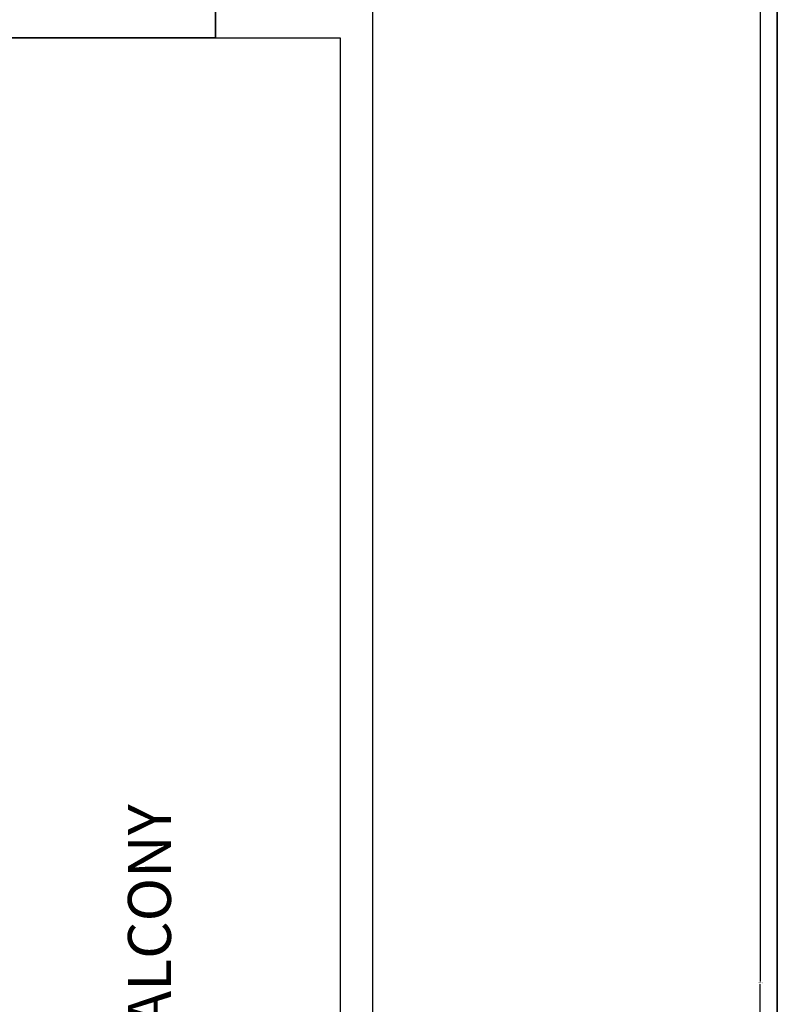
# Model space of a CAD drawing. Units: inches. Extents: x 1088 to 1703, y 668 to 1875.
# Tile 40 of 45: x 1598 to 1703, y 1606 to 1743. Entities that reach past the tile are written whole.
import ezdxf

# ---------------------------------------------------------------- set-up
doc = ezdxf.new("R2010")
doc.units = ezdxf.units.IN
for name, color, linetype, lineweight in [('A-ANNO-DIMS', 2, 'Continuous', 18), ('A-ANNO-TTLB', 7, 'Continuous', 35), ('A-AREA-IDEN', 7, 'Continuous', 18), ('A-FLOR-HRAL', 7, 'Continuous', 25), ('A-WALL', 7, 'Continuous', 35)]:
    doc.layers.add(name, color=color, linetype=linetype, lineweight=lineweight)
doc.styles.get("Standard").update_dxf_attribs({"font": 'arial.ttf'})
doc.dimstyles.get("Standard").update_dxf_attribs({"dimtxt": 0.18, "dimasz": 0.18, "dimexe": 0.18, "dimexo": 0.0625, "dimgap": 0.09, "dimtad": 0, "dimtih": 1, "dimtoh": 1, "dimdec": 4, "dimzin": 0, "dimdsep": 46, "dimtxsty": 'Standard', "dimcen": 0.09, "dimadec": 0, "dimazin": 0, "dimtfac": 1, "dimtdec": 4, "dimtofl": 0, "dimtmove": 0, "dimatfit": 3, "dimfxl": 1, "dimtolj": 1, "dimtzin": 0, "dimarcsym": 0})

# ---------------------------------------------------------------- blocks, each defined once
blk = doc.blocks.new('*D30')
at = {"layer": 'A-ANNO-DIMS', "color": 0, "lineweight": -2, "transparency": 16777216}
for p, q in [((1624.91, 1803.56), (1700.97, 1803.56)), ((1700.79, 1803.38), (1700.79, 1609.49)), ((1700.79, 1415.24), (1700.79, 1609.13)), ((1620.41, 1415.06), (1700.97, 1415.06))]:
    blk.add_line(p, q, dxfattribs=at)
at = {"layer": 'A-ANNO-DIMS', "color": 0, "transparency": 16777216}
for points in [[(1700.76, 1803.38), (1700.82, 1803.38), (1700.79, 1803.56)], [(1700.76, 1415.24), (1700.82, 1415.24), (1700.79, 1415.06)]]:
    blk.add_solid(points, dxfattribs=at)
at = {"layer": 'Defpoints', "color": 0, "transparency": 16777216}
for p in [(1624.84, 1803.56), (1700.79, 1803.56), (1620.34, 1415.06)]:
    blk.add_point(p, dxfattribs=at)
at = {"layer": 'A-ANNO-DIMS', "color": 0, "transparency": 16777216, "insert": (1700.79, 1609.31), "char_height": 0.18, "attachment_point": 5}
blk.add_mtext('\\A1;388.5', dxfattribs=at)

msp = doc.modelspace()

# ---------------------------------------------------------------- linework, layer by layer
at = {"layer": 'A-ANNO-TTLB'}
msp.add_lwpolyline([(1088.369, 1874.677), (1703.181, 1874.677), (1703.181, 667.947), (1088.369, 667.947)], close=True, dxfattribs=at)
at = {"layer": 'A-FLOR-HRAL'}
for p, q in [((1646.743, 1745.49), (1646.743, 1474.363)), ((1624.845, 1740.99), (1642.243, 1740.99)), ((1642.243, 1740.99), (1642.243, 1474.363))]:
    msp.add_line(p, q, dxfattribs=at)
at = {"layer": 'A-WALL'}
for p, q in [((1624.845, 1803.558), (1624.845, 1740.99)), ((1620.345, 1740.99), (1590.345, 1740.99)), ((1620.345, 1740.99), (1624.845, 1740.99))]:
    msp.add_line(p, q, dxfattribs=at)

# ---------------------------------------------------------------- texts
at = {"layer": 'A-AREA-IDEN', "insert": (1612.649, 1558.891), "char_height": 6, "attachment_point": 1, "rotation": 90}
msp.add_mtext_dynamic_manual_height_columns('3\'6" WIDE BALCONY', width=280.65936, gutter_width=12.5, heights=[0], dxfattribs=at)

# ---------------------------------------------------------------- dimensions: what is measured, and where the dimension line sits
at = {"layer": 'A-ANNO-DIMS'}
dim = msp.add_linear_dim(base=(1700.793, 1803.558), p1=(1620.345, 1415.058), p2=(1624.845, 1803.558), angle=90, dimstyle='Standard', override={"dimdec": 1, "dimlfac": 1, "dimrnd": 0, "dimzin": 0, "dimdsep": 46, "dimlunit": 2}, dxfattribs=at)
dim.commit()
dim.dimension.update_dxf_attribs({"geometry": '*D30', "text_midpoint": (1700.793, 1609.308)})

doc.saveas('drawing.dxf')
